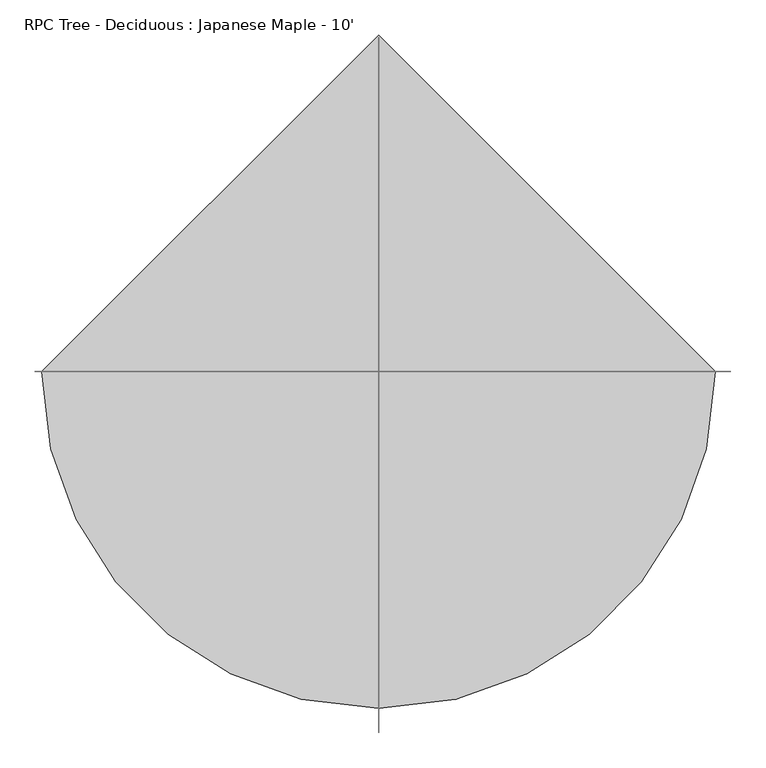
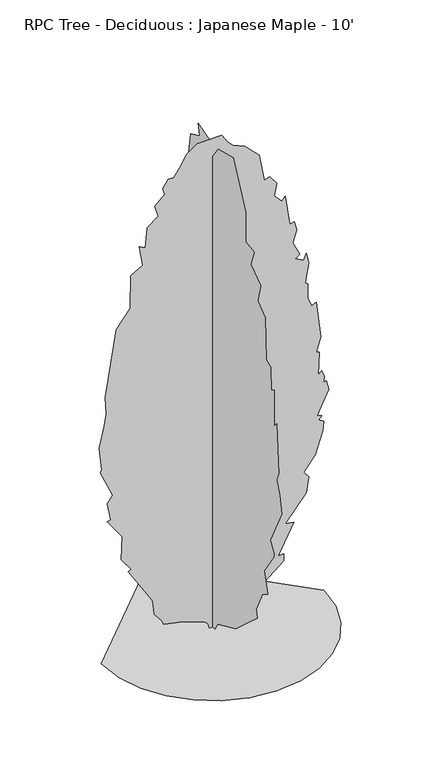
"""IFC4 building model written with IfcOpenShell, lengths in millimetres: geographic element geometry, RPC Tree - Deciduous : Japanese Maple - 10'."""

from ifc_helpers import new_model, si_unit, origin, place, context, project, spatial, triangles, source, transform, mapped, element, save


def rpc_tree_deciduous_japanese_maple_10_8b15208c(model_context):
    return source(origin(), model_context, "Body", "Tessellation", [
        triangles([(-21.0204534, 9e-07, 1.9e-06), (-26.0054008, -4e-07, 25.6281368), (-39.4557585, -9e-07, 43.4163588), (-176.807431, 2.1e-06, 93.9654218), (-288.3896281, 5.6e-06, 117.6426557), (-299.0845058, 4.5e-06, 144.3795048), (-342.1757346, 3.1e-06, 199.5412178), (-352.5589308, -1.5e-06, 283.4115708), (-368.6023556, -2.7e-06, 315.4958588), (-496.9380904, -9.2e-06, 518.6950473), (-480.3336897, -1.05e-05, 528.6736533), (-537.1173603, -1.28e-05, 608.2775153), (-531.3624427, -2.14e-05, 749.4692968), (-619.9288754, -2.49e-05, 871.625576), (-598.5383932, -2.61e-05, 876.9704533), (-619.0979668, -3.17e-05, 985.0297005), (-587.8413354, -3.55e-05, 1026.6967066), (-662.7062788, -4.21e-05, 1192.4684921), (-652.0128181, -4.32e-05, 1203.1619528), (-668.0547895, -5.11e-05, 1347.5396954), (-639.0333778, -5.99e-05, 1473.5058437), (-625.2738253, -6.48e-05, 1545.395351), (-630.622336, -7.06e-05, 1646.9956902), (-566.4544868, -9.73e-05, 2048.0485359), (-486.2446298, -0.0001072, 2154.9973858), (-481.9084846, -0.0001193, 2354.6093296), (-411.3797227, -0.0001248, 2395.6303722), (-432.7702048, -0.0001312, 2518.6174873), (-396.2630219, -0.0001316, 2497.6734169), (-384.644327, -0.0001394, 2620.2179718), (-320.4738979, -0.000145, 2668.3438133), (-341.8636897, -0.0001482, 2737.8602097), (-283.0421711, -0.000154, 2791.3345619), (-293.737067, -0.0001558, 2828.7671608), (-261.6527608, -0.00016, 2876.8930023), (-229.5684729, -0.0001614, 2876.8930023), (-192.7564938, -0.0001659, 2924.6886314), (-155.8509158, -0.0001716, 2994.0672455), (-89.6361621, -0.0001772, 3038.905497), (52.7396406, -0.0001836, 3041.1446045), (85.9273859, -0.0001819, 2989.1867294), (118.011683, -0.0001814, 2957.102932), (189.3441839, -0.0001827, 2926.891404), (273.0857112, -0.0001812, 2839.4606941), (305.1699992, -0.0001727, 2673.6923241), (337.2543054, -0.0001747, 2684.3858574), (376.3856741, -0.0001731, 2628.4041), (363.9904278, -0.0001683, 2556.0500862), (406.7714284, -0.0001673, 2507.9242447), (428.158277, -0.0001695, 2529.3147995), (454.8973063, -0.0001598, 2347.5008972), (481.632702, -0.0001613, 2352.849408), (496.1724395, -0.0001588, 2299.8757519), (472.2745886, -0.0001534, 2227.184404), (513.7166448, -0.0001499, 2138.9553417), (485.6967344, -0.0001477, 2122.1550591), (535.1071269, -0.0001483, 2096.1743774), (551.1490983, -0.0001513, 2133.606831), (567.1910697, -0.0001481, 2069.4389454), (545.8042211, -0.0001402, 1951.7967075), (561.243831, -0.0001401, 1939.0929771), (559.0993398, -0.0001348, 1852.232), (583.2330411, -0.0001326, 1796.7218708), (609.9720703, -0.0001344, 1807.4154041), (636.7074297, -0.0001222, 1582.8278046), (609.9720703, -0.0001159, 1497.2695095), (626.6235975, -0.0001163, 1491.6125874), (620.665531, -0.0001078, 1352.8882061), (642.0560131, -0.0001097, 1368.9301048), (658.0979845, -0.0001081, 1331.4976513), (652.7494011, -0.0001057, 1294.0688313), (668.7913725, -0.0001067, 1299.4137085), (684.8333439, -0.0001039, 1240.5943336), (615.3169476, -9.26e-05, 1101.5616137), (642.0560131, -9.31e-05, 1090.868153), (626.0140417, -9.11e-05, 1069.4776709), (652.7494011, -9.13e-05, 1053.4356995), (647.1251078, -8.76e-05, 995.8029528), (604.6235232, -7.77e-05, 860.9284819), (535.1071269, -6.96e-05, 775.3701141), (567.1910697, -6.88e-05, 737.9376606), (549.6541314, -6.24e-05, 644.5234497), (428.158277, -4.8e-05, 491.9596516), (476.2878247, -4.98e-05, 486.6111408), (385.3809099, -3.53e-05, 310.1484017), (417.4648527, -3.67e-05, 310.1484017), (417.4648527, -3.42e-05, 267.369236), (182.1795413, -1.24e-05, 74.8634718), (182.1795413, -1.4e-05, 101.600321), (21.7586533, -1e-06, 0.0), (1.5e-06, 19.6988158, 0.0001857), (3.7e-06, 49.2587393, 20.4233355), (7.3e-06, 110.6042953, 42.7795427), (1.03e-05, 254.9838002, 96.2532454), (1.66e-05, 329.847272, 165.7692784), (1.54e-05, 297.762984, 171.1167173), (2.76e-05, 412.2070341, 336.0808305), (2.97e-05, 377.9749666, 417.0947445), (3.42e-05, 474.2267587, 556.1275372), (3.65e-05, 463.5333344, 620.2953501), (4.33e-05, 533.0460972, 705.8537178), (4.88e-05, 556.4178174, 808.187079), (4.72e-05, 543.743155, 914.4029068), (5.65e-05, 629.3015591, 1042.738678), (6.24e-05, 634.6464363, 1171.07801), (6.56e-05, 603.7599495, 1276.1036488), (6.92e-05, 650.6884077, 1443.7950119), (6.99e-05, 607.9110406, 1502.6143867), (7.51e-05, 554.4366157, 1673.7311222), (7.61e-05, 591.8690692, 1791.3733601), (8.17e-05, 549.0880686, 1962.4900955), (8.38e-05, 495.6172771, 2064.0904346), (8.63e-05, 468.8782479, 2277.9881344), (8.42e-05, 436.7943051, 2261.9462357), (9.26e-05, 436.7943051, 2454.4498924), (9.05e-05, 372.6264559, 2470.4916458), (8.83e-05, 338.6788914, 2584.7195572), (9.15e-05, 319.1523943, 2679.0408348), (9.15e-05, 254.9838002, 2743.2087204), (9.86e-05, 222.899494, 2935.7158653), (9.07e-05, 131.9936965, 2978.4934868), (9.43e-05, 145.7997306, 3047.3276573), (8.69e-05, 16.2125085, 3006.0162254), (8.83e-05, 9.0039295, 2914.3256012), (8.37e-05, -55.1646243, 3005.2322617), (7.88e-05, -210.2386571, 3048.0098831), (6.75e-05, -338.5761724, 2785.9860512), (5.95e-05, -338.5761724, 2604.1759277), (5.52e-05, -423.1508429, 2589.1210327), (5.25e-05, -386.7017232, 2491.8822006), (5.07e-05, -489.7752645, 2421.5203617), (4.7e-05, -461.5666666, 2310.0720772), (4.12e-05, -536.4279402, 2251.2490688), (3.52e-05, -547.124998, 1994.5740383), (3.25e-05, -590.7841063, 1975.9485764), (2.61e-05, -595.2509122, 1834.1543243), (2.56e-05, -627.3348186, 1855.5412457), (2.16e-05, -627.3348186, 1630.9537914), (1.61e-05, -654.0702507, 1663.0377342), (7.8e-06, -675.4607328, 1363.5852276), (6.6e-06, -652.2414379, 1312.6508366), (1.7e-06, -686.157827, 1235.2458229), (2.1e-06, -702.1997257, 1128.2970457), (-3.1e-06, -589.9023651, 898.3609354), (-7.5e-06, -627.3348186, 834.1931225), (-2.6e-06, -624.1706949, 811.539854), (-4.6e-06, -525.7345159, 668.4248978), (-1.16e-05, -563.1669694, 545.4340765), (-1.07e-05, -504.3439974, 508.001623), (-8e-06, -445.5246952, 379.6658881), (-1.05e-05, -456.2181195, 331.5381935), (-1.01e-05, -349.2707231, 235.2853114), (-9.6e-06, -236.9755062, 133.6849814), (-5.2e-06, -49.8164542, 48.1266227), (-4e-07, -23.0802909, 0.0001832), (-654.5201506, 0.0, 0.0002131), (-637.2154655, -149.9726046, 0.0002035), (-587.9356974, -287.6987364, 0.0001931), (-510.625082, -409.231598, 0.0001825), (-409.231598, -510.625082, 0.000172), (-287.6987364, -587.9356974, 0.0001621), (-149.9726046, -637.2154655, 0.0001531), (2.94e-05, -654.5201506, 0.0001455), (149.9726046, -637.2154655, 0.00014), (287.6987364, -587.9356974, 0.0001369), (409.231598, -510.625082, 0.0001362), (510.625082, -409.231598, 0.0001378), (587.9356974, -287.6983731, 0.0001417), (637.2154655, -149.9726046, 0.0001477), (654.5201506, 5.72e-05, 0.0001559), (-8.55e-05, 654.5201506, 0.0002236)], [[57, 58, 59], [27, 28, 29], [87, 88, 89], [49, 50, 51], [13, 14, 15], [83, 84, 85], [74, 75, 76], [63, 64, 65], [68, 69, 70], [71, 72, 73], [9, 10, 11], [85, 86, 87], [85, 87, 89], [51, 52, 53], [54, 55, 56], [90, 1, 2], [66, 67, 68], [45, 46, 47], [17, 18, 19], [68, 70, 71], [45, 47, 48], [31, 32, 33], [76, 77, 78], [89, 90, 2], [89, 2, 3], [57, 59, 60], [51, 53, 54], [25, 26, 27], [39, 40, 41], [56, 57, 60], [71, 73, 74], [34, 35, 36], [33, 34, 36], [4, 5, 6], [60, 61, 62], [80, 81, 82], [38, 39, 41], [37, 38, 41], [37, 41, 42], [29, 30, 31], [15, 16, 17], [36, 37, 42], [33, 36, 42], [31, 33, 42], [31, 42, 43], [31, 43, 44], [31, 44, 45], [29, 31, 45], [29, 45, 48], [27, 29, 48], [25, 27, 48], [25, 48, 49], [25, 49, 51], [25, 51, 54], [25, 54, 56], [25, 56, 60], [25, 60, 62], [24, 25, 62], [23, 24, 62], [22, 23, 62], [22, 62, 63], [22, 63, 65], [22, 65, 66], [22, 66, 68], [21, 22, 68], [20, 21, 68], [19, 20, 68], [17, 19, 68], [17, 68, 71], [17, 71, 74], [15, 17, 74], [13, 15, 74], [13, 74, 76], [13, 76, 78], [13, 78, 79], [13, 79, 80], [12, 13, 80], [11, 12, 80], [9, 11, 80], [9, 80, 82], [9, 82, 83], [9, 83, 85], [9, 85, 89], [9, 89, 3], [9, 3, 4], [8, 9, 4], [8, 4, 6], [7, 8, 6], [138, 139, 140], [94, 95, 96], [136, 137, 138], [121, 122, 123], [112, 113, 114], [128, 129, 130], [121, 123, 124], [125, 126, 127], [124, 125, 127], [114, 115, 116], [147, 148, 149], [130, 131, 132], [124, 127, 128], [134, 135, 136], [154, 155, 91], [154, 91, 92], [150, 151, 152], [96, 97, 98], [119, 120, 121], [119, 121, 124], [119, 124, 128], [118, 119, 128], [117, 118, 128], [116, 117, 128], [116, 128, 130], [114, 116, 130], [114, 130, 132], [112, 114, 132], [112, 132, 133], [112, 133, 134], [112, 134, 136], [111, 112, 136], [110, 111, 136], [109, 110, 136], [109, 136, 138], [109, 138, 140], [109, 140, 141], [108, 109, 141], [107, 108, 141], [106, 107, 141], [105, 106, 141], [104, 105, 141], [103, 104, 141], [103, 141, 142], [103, 142, 143], [103, 143, 144], [102, 103, 144], [101, 102, 144], [100, 101, 144], [100, 144, 145], [100, 145, 146], [100, 146, 147], [100, 147, 149], [100, 149, 150], [100, 150, 152], [100, 152, 153], [100, 153, 154], [99, 100, 154], [98, 99, 154], [96, 98, 154], [96, 154, 92], [96, 92, 93], [96, 93, 94], [170, 171, 156], [169, 170, 156], [169, 156, 157], [168, 169, 157], [168, 157, 158], [168, 158, 159], [167, 168, 159], [166, 167, 159], [166, 159, 160], [166, 160, 161], [166, 161, 162], [166, 162, 163], [166, 163, 164], [166, 164, 165]], closed=False),
    ])


if __name__ == "__main__":
    model = new_model("IFC4")
    model_context = context("Model", 3, world=origin())
    ifc_project = project(units=[si_unit("LENGTHUNIT", "METRE", prefix="MILLI")], contexts=[model_context])
    site = spatial("IfcSite", under=ifc_project)
    building = spatial("IfcBuilding", under=site)
    placement = place(None, origin())
    rpc_tree_deciduous_japanese_maple_10_shape = rpc_tree_deciduous_japanese_maple_10_8b15208c(model_context)
    element("IfcGeographicElement", 1, ObjectType="RPC Tree - Deciduous : Japanese Maple - 10'", at=placement, inside=building, context=model_context, shape_type="MappedRepresentation", body=[
        mapped(rpc_tree_deciduous_japanese_maple_10_shape, transform((0.0, 0.0, 0.0), x_axis=(1.0, 0.0, 0.0), y_axis=(0.0, 1.0, 0.0), z_axis=(0.0, 0.0, 1.0))),
    ])
    save(model, "model.ifc")

# Revit data of these elements
# Type "RPC Tree - Deciduous : Japanese Maple - 10'"
#   built-in parameter 1005195 = "RPC-16-FUM3-UUQ0-UBF0-N000-ST1L-LVER-AU"
#   Type Comments = "Japanese Maple"
#   Assembly Code = "G2050500"
#   Height = 10' - 0"
#   Default Elevation = 0
